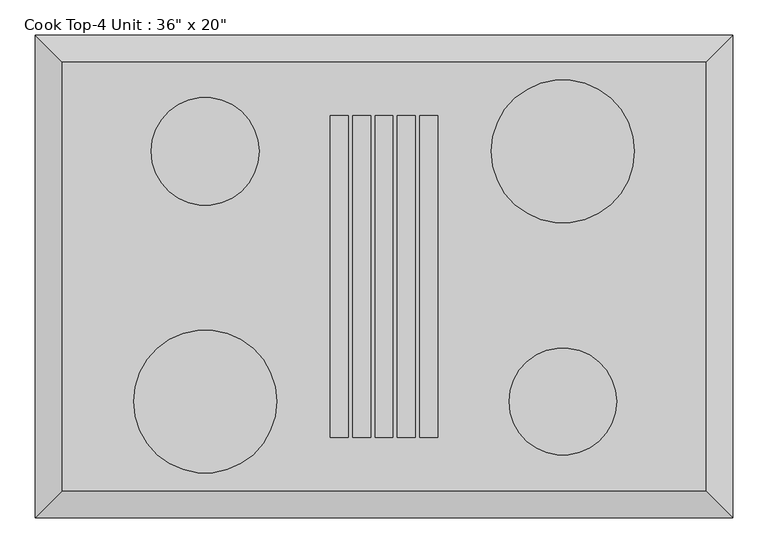
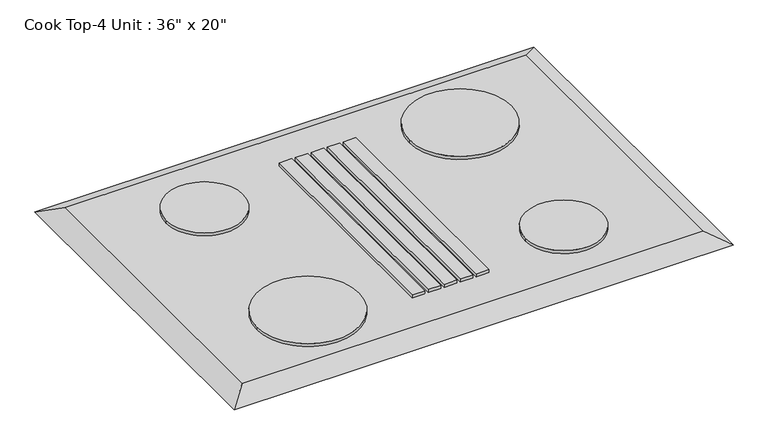
"""IFC4 building model written with IfcOpenShell, lengths in millimetres: proxy geometry."""

from ifc_helpers import new_model, si_unit, point, frame, frame_2d, origin, place, context, project, spatial, polyline, circle_curve, trimmed, segment, composite_curve, outline, extrude, faceted_brep, source, transform, mapped, element, save


def proxy_bb1e6e30(model_context):
    return source(origin(), model_context, "Body", "SolidModel", [
        extrude(outline(composite_curve([segment(trimmed(circle_curve(frame_2d((-254.0, 177.8)), 76.5869489), [point((-177.4130511, 177.8))], [point((-330.5869489, 177.8))], False, "CARTESIAN"), True, "CONTINUOUS"), segment(trimmed(circle_curve(frame_2d((-254.0, 177.8)), 76.5869489), [point((-330.5869489, 177.8))], [point((-177.4130511, 177.8))], False, "CARTESIAN"), True, "CONTINUOUS")], self_intersect=False)), frame((0.0, 0.0, 806.45), z_axis=(0.0, 0.0, 1.0), x_axis=(1.0, 0.0, 0.0)), (0.0, 0.0, 1.0), 6.35),
        extrude(outline(composite_curve([segment(trimmed(circle_curve(frame_2d((254.0, 177.8)), 101.6), [point((355.6, 177.8))], [point((152.4, 177.8))], False, "CARTESIAN"), True, "CONTINUOUS"), segment(trimmed(circle_curve(frame_2d((254.0, 177.8)), 101.6), [point((152.4, 177.8))], [point((355.6, 177.8))], False, "CARTESIAN"), True, "CONTINUOUS")], self_intersect=False)), frame((0.0, 0.0, 806.45), z_axis=(0.0, 0.0, 1.0), x_axis=(1.0, 0.0, 0.0)), (0.0, 0.0, 1.0), 6.35),
        extrude(outline(composite_curve([segment(trimmed(circle_curve(frame_2d((254.0, -177.8)), 76.2), [point((330.2, -177.8))], [point((177.8, -177.8))], False, "CARTESIAN"), True, "CONTINUOUS"), segment(trimmed(circle_curve(frame_2d((254.0, -177.8)), 76.2), [point((177.8, -177.8))], [point((330.2, -177.8))], False, "CARTESIAN"), True, "CONTINUOUS")], self_intersect=False)), frame((0.0, 0.0, 806.45), z_axis=(0.0, 0.0, 1.0), x_axis=(1.0, 0.0, 0.0)), (0.0, 0.0, 1.0), 6.35),
        extrude(outline(polyline([(-50.8, 228.6), (-50.8, -228.6), (-76.2, -228.6), (-76.2, 228.6), (-50.8, 228.6)])), frame((0.0, 0.0, 806.45), z_axis=(0.0, 0.0, 1.0), x_axis=(1.0, 0.0, 0.0)), (0.0, 0.0, 1.0), 6.35),
        extrude(outline(polyline([(-19.05, 228.6), (-19.05, -228.6), (-44.45, -228.6), (-44.45, 228.6), (-19.05, 228.6)])), frame((0.0, 0.0, 806.45), z_axis=(0.0, 0.0, 1.0), x_axis=(1.0, 0.0, 0.0)), (0.0, 0.0, 1.0), 6.35),
        extrude(outline(polyline([(12.7, 228.6), (12.7, -228.6), (-12.7, -228.6), (-12.7, 228.6), (12.7, 228.6)])), frame((0.0, 0.0, 806.45), z_axis=(0.0, 0.0, 1.0), x_axis=(1.0, 0.0, 0.0)), (0.0, 0.0, 1.0), 6.35),
        extrude(outline(polyline([(44.45, 228.6), (44.45, -228.6), (19.05, -228.6), (19.05, 228.6), (44.45, 228.6)])), frame((0.0, 0.0, 806.45), z_axis=(0.0, 0.0, 1.0), x_axis=(1.0, 0.0, 0.0)), (0.0, 0.0, 1.0), 6.35),
        extrude(outline(polyline([(76.2, 228.6), (76.2, -228.6), (50.8, -228.6), (50.8, 228.6), (76.2, 228.6)])), frame((0.0, 0.0, 806.45), z_axis=(0.0, 0.0, 1.0), x_axis=(1.0, 0.0, 0.0)), (0.0, 0.0, 1.0), 6.35),
        faceted_brep([(457.2, 304.8, 806.45), (-457.2, 304.8, 806.45), (-457.2, -304.8, 806.45), (457.2, -304.8, 806.45), (495.3, 342.9, 787.4), (495.3, -342.9, 787.4), (-495.3, -342.9, 787.4), (-495.3, 342.9, 787.4)], [[[0, 1, 2, 3]], [[4, 5, 6, 7]], [[4, 7, 1, 0]], [[7, 6, 2, 1]], [[6, 5, 3, 2]], [[5, 4, 0, 3]]]),
        extrude(outline(composite_curve([segment(trimmed(circle_curve(frame_2d((-254.0, -177.8)), 101.6), [point((-152.4, -177.8))], [point((-355.6, -177.8))], False, "CARTESIAN"), True, "CONTINUOUS"), segment(trimmed(circle_curve(frame_2d((-254.0, -177.8)), 101.6), [point((-355.6, -177.8))], [point((-152.4, -177.8))], False, "CARTESIAN"), True, "CONTINUOUS")], self_intersect=False)), frame((0.0, 0.0, 806.45), z_axis=(0.0, 0.0, 1.0), x_axis=(1.0, 0.0, 0.0)), (0.0, 0.0, 1.0), 6.35),
    ])


if __name__ == "__main__":
    model = new_model("IFC4")
    model_context = context("Model", 3, world=origin())
    ifc_project = project(units=[si_unit("LENGTHUNIT", "METRE", prefix="MILLI")], contexts=[model_context])
    site = spatial("IfcSite", under=ifc_project)
    building = spatial("IfcBuilding", under=site)
    placement = place(None, origin())
    proxy_shape = proxy_bb1e6e30(model_context)
    element("IfcBuildingElementProxy", 1, Name="Cook Top-4 Unit : 36\" x 20\"", ObjectType="Cook Top-4 Unit : 36\" x 20\"", at=placement, inside=building, context=model_context, shape_type="MappedRepresentation", body=[
        mapped(proxy_shape, transform((0.0, 0.0, 0.0), x_axis=(1.0, 0.0, 0.0), y_axis=(0.0, 1.0, 0.0), z_axis=(0.0, 0.0, 1.0))),
    ])
    save(model, "model.ifc")

# Revit data of these elements
# Type "Cook Top-4 Unit : 36\" x 20\""
#   Assembly Code = "E1090400"
#   Depth = 2' - 0"
#   Width = 3' - 0"
#   Burner Material = Steel, Chrome Plated
#   Cooktop Material = Steel, Polished
#   Default Elevation = 0
# Element 1 (IfcBuildingElementProxy, "Cook Top-4 Unit : 36\" x 20\"")
#   Materials on its faces: "Steel, Chrome Plated", "Steel, Polished"
# Materials
#   "Steel, Chrome Plated": class "Metal", colour RGB 17 17 17, transparency 0, Description = "Chromiuim plated steel", Cost = 0
#   "Steel, Polished": class "Metal", colour RGB 57 57 57, transparency 0, Description = "Polished steel", Cost = 0
